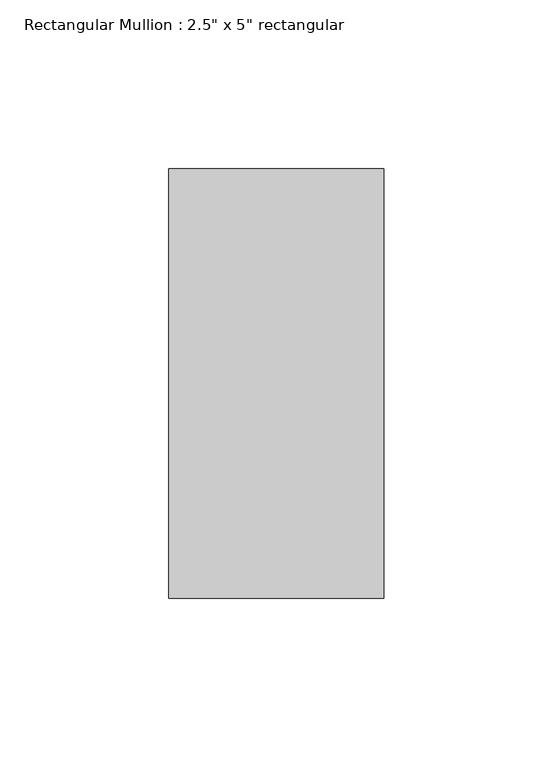
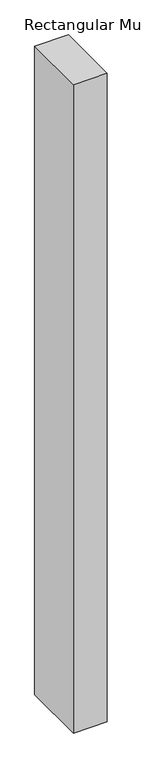
"""IFC4 building model written with IfcOpenShell, lengths in millimetres: member geometry."""

from ifc_helpers import new_model, si_unit, frame, origin, place, context, project, spatial, polyline, outline, extrude, source, transform, mapped, element, save


def member_547128e5(model_context):
    return source(origin(), model_context, "Body", "SweptSolid", [
        extrude(outline(polyline([(0.0, 63.5), (0.0, -63.5), (-63.5, -63.5), (-63.5, 63.5), (0.0, 63.5)])), frame((0.0, 0.0, -1295.4), z_axis=(0.0, 0.0, 1.0), x_axis=(1.0, 0.0, 0.0)), (0.0, 0.0, 1.0), 1295.4),
    ])


if __name__ == "__main__":
    model = new_model("IFC4")
    model_context = context("Model", 3, world=origin())
    ifc_project = project(units=[si_unit("LENGTHUNIT", "METRE", prefix="MILLI")], contexts=[model_context])
    site = spatial("IfcSite", under=ifc_project)
    building = spatial("IfcBuilding", under=site)
    placement = place(None, origin())
    member_shape = member_547128e5(model_context)
    element("IfcMember", 1, ObjectType="Rectangular Mullion : 2.5\" x 5\" rectangular", at=placement, inside=building, context=model_context, shape_type="MappedRepresentation", body=[
        mapped(member_shape, transform((0.0, 0.0, 0.0), x_axis=(1.0, 0.0, 0.0), y_axis=(0.0, 1.0, 0.0), z_axis=(0.0, 0.0, 1.0))),
    ])
    save(model, "model.ifc")

# Revit data of these elements
# Type "Rectangular Mullion : 2.5\" x 5\" rectangular"
#   built-in parameter 1007304 = 0.416667 (stored number, unit not read)
#   built-in parameter 1007301 = 0.104167 (stored number, unit not read)
#   built-in parameter 1007300 = 0.104167 (stored number, unit not read)
# Element 1 (IfcMember, "Rectangular Mullion : 2.5\" x 5\" rectangular")
#   Materials on its faces: "Aluminum"
# Materials
#   "Aluminum": class "Metal", colour RGB 247 247 247, transparency 0, Description = "Aluminum 6061", Cost = 0
